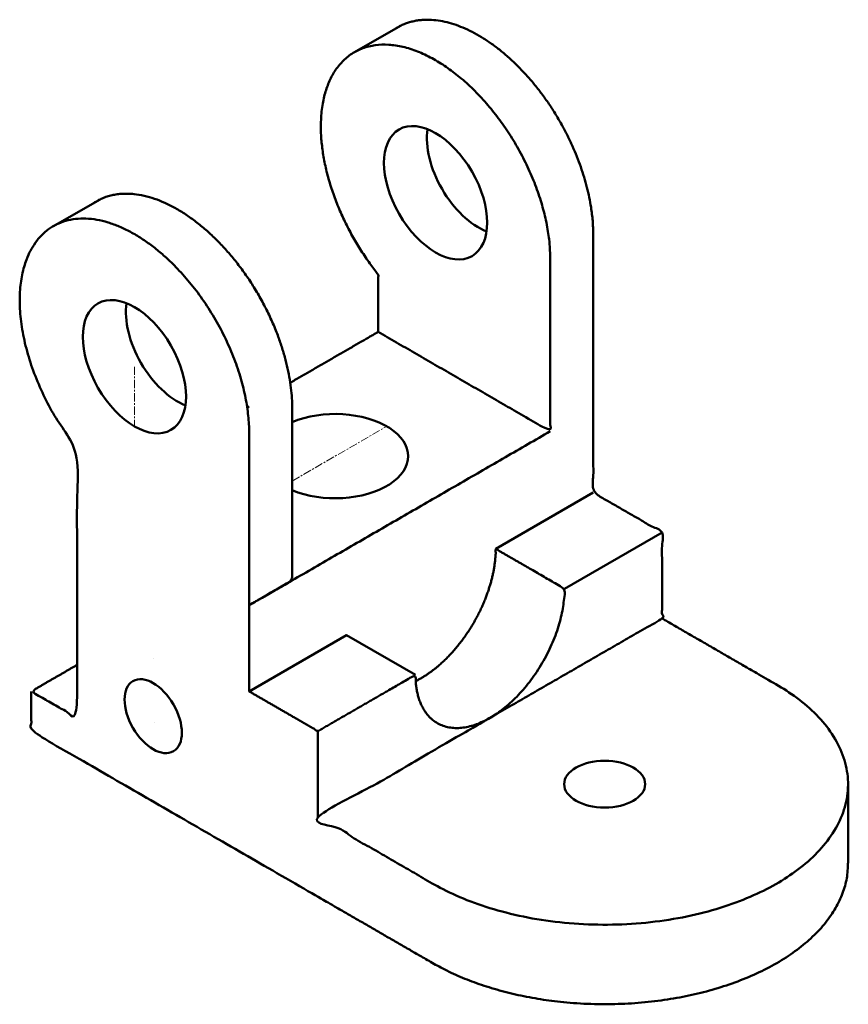
# Model space of a CAD drawing. Units: millimetres. Extents: x -23 to 102, y 22 to 171.
import ezdxf

# ---------------------------------------------------------------- set-up
doc = ezdxf.new("R2010")
doc.units = ezdxf.units.MM
doc.header["$MEASUREMENT"] = 0
doc.linetypes.add('CENTER', pattern=[2, 1.25, -0.25, 0.25, -0.25])
doc.layers.add('M-CNTR', color=1, linetype='CENTER', lineweight=18)
doc.layers.add('M-OUTL', color=7, linetype='Continuous', lineweight=50)

msp = doc.modelspace()

# ---------------------------------------------------------------- linework, layer by layer
at = {"layer": 'M-CNTR'}
for p, q in [((-6.06, 118.32), (-6.06, 109.32)), ((17.76, 101.07), (32.05, 109.32)), ((-3.03, 64.57), (-3.03, 64.57))]:
    msp.add_line(p, q, dxfattribs=at)
msp.add_lwpolyline([(-3.18, 74.32), (-3.18, 74.32)], close=True, dxfattribs=at)
at = {"layer": 'M-OUTL'}
for p, q in [((34.1, 169.77), (27.17, 165.79)), ((-11.36, 143.52), (-18.29, 139.54)), ((11.26, 112.32), (10.97, 112.15)), ((48.5, 90.82), (63.22, 99.32)), ((58.89, 84.82), (73.62, 93.32)), ((21.65, 50.32), (21.65, 63.32))]:
    msp.add_line(p, q, dxfattribs=at)
msp.add_lwpolyline([(11.26, 69.32), (25.98, 77.82), (36.38, 71.82)], dxfattribs=at)
for centre, major_axis in [((39.41, 144.57), (5.51, -9.55)), ((-6.06, 118.32), (5.51, -9.55)), ((-3.23, 65.58), (3.06, -5.3)), ((64.95, 55.32), (-6.12, 0))]:
    msp.add_ellipse(centre, major_axis=major_axis, ratio=0.57735, dxfattribs=at)
for centre, major_axis, start_param, end_param in [((45.9, 148.32), (5.51, -9.55), 3.77173, 5.653048), ((0.44, 122.07), (5.51, -9.55), 3.77173, 5.653048), ((24.25, 104.82), (-11.02, 0), 0.940659, 5.342526)]:
    msp.add_ellipse(centre, major_axis=major_axis, ratio=0.57735, start_param=start_param, end_param=end_param, dxfattribs=at)
for points, weights, knots in [([(73.62, 80.32), (82.28, 75.32), (90.94, 70.32), (116.92, 55.32), (90.94, 40.32), (64.95, 25.32), (38.97, 40.32), (30.31, 45.32), (21.65, 50.32), (47.63, 65.32), (73.62, 80.32), (73.62, 86.82), (73.62, 93.32), (68.42, 96.32), (63.22, 99.32), (63.22, 105.82), (63.22, 112.32), (63.22, 115.32), (63.22, 118.32), (63.22, 128.32), (63.22, 138.32), (63.22, 151.93), (52.26, 163.25), (41.3, 174.58), (33.25, 169.28)], [1, 1, 1, 0.707106781187, 1, 0.707106781187, 1, 1, 1, 1, 1, 1, 1, 1, 1, 1, 1, 1, 1, 1, 1, 0.826761759284, 1, 0.826761759284, 1], [0, 0, 0, 1, 1, 2.570796, 2.570796, 4.141593, 4.141593, 5.141593, 5.141593, 6.141593, 6.141593, 7.141593, 7.141593, 8.141593, 8.141593, 9.141593, 9.141593, 10.141593, 10.141593, 11.141593, 11.141593, 12.336532, 12.336532, 13.531471, 13.531471, 13.531471]), ([(30.75, 123.57), (43.74, 116.07), (56.73, 108.57), (56.73, 111.57), (56.73, 114.57), (56.73, 124.57), (56.73, 134.57), (56.73, 151.35), (42.41, 162.53), (28.1, 173.71), (23.13, 160.81), (18.16, 147.91), (30.75, 132.25), (30.75, 130.91), (30.75, 129.57), (30.75, 126.57), (30.75, 123.57), (24.11, 119.74), (17.46, 115.9)], [1, 1, 1, 1, 1, 1, 1, 0.766044443119, 1, 0.766044443119, 1, 0.766044443119, 1, 1, 1, 1, 1, 1, 1], [0, 0, 0, 1, 1, 2, 2, 3, 3, 4.396263, 4.396263, 5.792527, 5.792527, 7.18879, 7.18879, 8.18879, 8.18879, 9.18879, 9.18879, 10.18879, 10.18879, 10.18879]), ([(56.73, 108.57), (33.99, 95.45), (11.26, 82.32), (14.51, 84.2), (17.76, 86.07), (17.76, 89.07), (17.76, 92.07), (17.76, 102.07), (17.76, 112.07), (17.76, 125.68), (6.79, 137), (-4.17, 148.33), (-12.22, 143.03)], [1, 1, 1, 1, 1, 1, 1, 1, 1, 0.826761759284, 1, 0.826761759284, 1], [0, 0, 0, 1, 1, 2, 2, 3, 3, 4, 4, 5.194939, 5.194939, 6.389878, 6.389878, 6.389878]), ([(36.41, 70.87), (41.3, 73.28), (44.9, 79.22), (48.5, 85.15), (48.5, 90.82), (53.7, 87.82), (58.89, 84.82), (58.89, 71.82), (47.63, 65.32), (36.38, 58.82), (36.38, 71.82), (29.01, 67.57), (21.65, 63.32), (16.46, 66.32), (11.26, 69.32), (11.26, 75.82), (11.26, 82.32), (11.26, 85.32), (11.26, 88.32), (11.26, 98.32), (11.26, 108.32), (11.26, 125.1), (-3.05, 136.28), (-17.36, 147.46), (-22.34, 134.56), (-27.31, 121.66), (-14.72, 106), (-14.72, 85.66), (-14.72, 65.32), (-18.18, 67.32), (-21.65, 69.32), (-18.18, 71.32), (-14.72, 73.32)], [1, 0.916618519181, 1, 0.916618519181, 1, 1, 1, 0.707106781187, 1, 0.707106781187, 1, 1, 1, 1, 1, 1, 1, 1, 1, 1, 1, 0.766044443119, 1, 0.766044443119, 1, 0.766044443119, 1, 1, 1, 1, 1, 1, 1], [0, 0, 0, 0.822517, 0.822517, 1.645033, 1.645033, 2.645033, 2.645033, 4.21583, 4.21583, 5.786626, 5.786626, 6.786626, 6.786626, 7.786626, 7.786626, 8.786626, 8.786626, 9.786626, 9.786626, 10.786626, 10.786626, 12.182889, 12.182889, 13.579153, 13.579153, 14.975416, 14.975416, 15.975416, 15.975416, 16.975416, 16.975416, 17.975416, 17.975416, 17.975416]), ([(-21.65, 69.32), (-21.65, 66.32), (-21.65, 63.32), (0, 50.82), (21.65, 38.32), (30.31, 33.32), (38.97, 28.32), (56.33, 18.3), (79.02, 23.72), (101.7, 29.15), (101.7, 43.32), (101.7, 49.32), (101.7, 55.32)], [1, 1, 1, 1, 1, 1, 1, 0.831469612303, 1, 0.831469612303, 1, 1, 1], [0, 0, 0, 1, 1, 2, 2, 3, 3, 4.178097, 4.178097, 5.356194, 5.356194, 6.356194, 6.356194, 6.356194])]:
    msp.add_rational_spline(points, weights, degree=2, knots=knots, dxfattribs=at)

doc.saveas('drawing.dxf')
